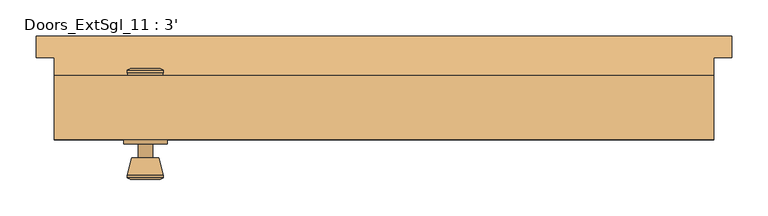
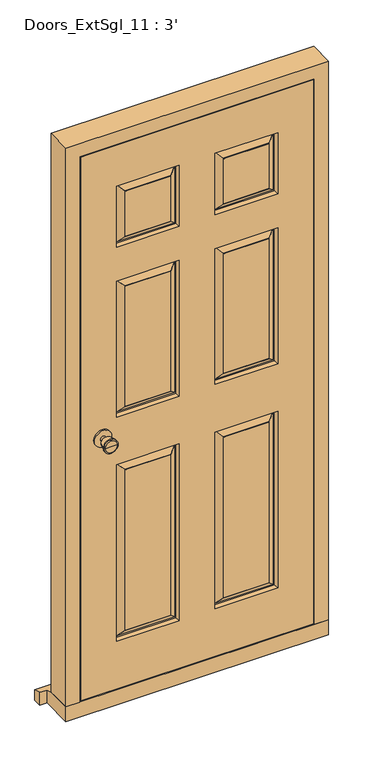
"""IFC4 building model written with IfcOpenShell, lengths in millimetres: door geometry, Doors_ExtSgl_11 : 3'."""

from ifc_helpers import new_model, si_unit, point, frame, frame_2d, origin, place, context, project, spatial, polyline, circle_curve, trimmed, segment, composite_curve, outline, extrude, faceted_brep, source, transform, mapped, element, save
from ifc_brep_helpers import plane_surface, cylinder_surface, revolved_surface, advanced_brep


def doors_extsgl_11_3_cb0934a6(model_context):
    return source(origin(), model_context, "Body", "SolidModel", [
        advanced_brep(
        [(-330.7, -51.42, 1000.0), (-320.7, -51.42, 1000.0), (-340.7, -51.42, 1000.0), (-310.2241324, -100.42, 1000.0), (-330.7, -100.42, 1000.0), (-351.1758676, -100.42, 1000.0), (-305.7, -98.5921319, 1000.0), (-355.7, -98.5921319, 1000.0), (-305.7, -95.1284537, 1000.0), (-355.7, -95.1284537, 1000.0), (-312.063764, -70.42, 1000.0), (-349.336236, -70.42, 1000.0), (-320.7, -70.42, 1000.0), (-340.7, -70.42, 1000.0)],
        [
            (0, 1),
            (1, 2, circle_curve(frame((-330.7, -51.42, 1000.0), z_axis=(0.0, 1.0, 0.0), x_axis=(-1.0, 0.0, 0.0)), 10.0)),
            (2, 0),
            (2, 1, circle_curve(frame((-330.7, -51.42, 1000.0), z_axis=(0.0, 1.0, 0.0), x_axis=(-1.0, 0.0, 0.0)), 10.0)),
            (3, 4),
            (4, 5),
            (5, 3, circle_curve(frame((-330.7, -100.42, 1000.0), z_axis=(0.0, -1.0, 0.0), x_axis=(-1.0, 0.0, 0.0)), 20.4758676)),
            (3, 5, circle_curve(frame((-330.7, -100.42, 1000.0), z_axis=(0.0, -1.0, 0.0), x_axis=(-1.0, 0.0, 0.0)), 20.4758676)),
            (6, 3),
            (5, 7),
            (7, 6, circle_curve(frame((-330.7, -98.5921319, 1000.0), z_axis=(0.0, -1.0, 0.0), x_axis=(-1.0, 0.0, 0.0)), 25.0)),
            (6, 7, circle_curve(frame((-330.7, -98.5921319, 1000.0), z_axis=(0.0, -1.0, 0.0), x_axis=(-1.0, 0.0, 0.0)), 25.0)),
            (8, 6),
            (7, 9),
            (9, 8, circle_curve(frame((-330.7, -95.1284537, 1000.0), z_axis=(0.0, -1.0, 0.0), x_axis=(-1.0, 0.0, 0.0)), 25.0)),
            (8, 9, circle_curve(frame((-330.7, -95.1284537, 1000.0), z_axis=(0.0, -1.0, 0.0), x_axis=(-1.0, 0.0, 0.0)), 25.0)),
            (10, 8),
            (9, 11),
            (11, 10, circle_curve(frame((-330.7, -70.42, 1000.0), z_axis=(0.0, -1.0, 0.0), x_axis=(-1.0, 0.0, 0.0)), 18.636236)),
            (10, 11, circle_curve(frame((-330.7, -70.42, 1000.0), z_axis=(0.0, -1.0, 0.0), x_axis=(-1.0, 0.0, 0.0)), 18.636236)),
            (12, 10),
            (11, 13),
            (13, 12, circle_curve(frame((-330.7, -70.42, 1000.0), z_axis=(0.0, -1.0, 0.0), x_axis=(-1.0, 0.0, 0.0)), 10.0)),
            (12, 13, circle_curve(frame((-330.7, -70.42, 1000.0), z_axis=(0.0, -1.0, 0.0), x_axis=(-1.0, 0.0, 0.0)), 10.0)),
            (1, 12),
            (13, 2),
        ],
        [
            plane_surface(frame((-330.7, -51.42, 1000.0), z_axis=(0.0, 1.0, 0.0), x_axis=(-1.0, 0.0, 0.0))),
            plane_surface(frame((-330.7, -100.42, 1000.0), z_axis=(0.0, -1.0, 0.0), x_axis=(-1.0, 0.0, 0.0))),
            revolved_surface(polyline([(-351.1758676, -100.42, 1000.0), (-355.7, -98.5921319, 1000.0)]), (-330.7, -51.42, 1000.0), (0.0, 1.0, 0.0)),
            cylinder_surface(frame((-330.7, -51.42, 1000.0), z_axis=(0.0, 1.0, 0.0), x_axis=(-1.0, 0.0, 0.0)), 25.0),
            revolved_surface(polyline([(-355.7, -95.1284537, 1000.0), (-349.336236, -70.42, 1000.0)]), (-330.7, -51.42, 1000.0), (0.0, 1.0, 0.0)),
            plane_surface(frame((-330.7, -70.42, 1000.0), z_axis=(0.0, 1.0, 0.0), x_axis=(-1.0, 0.0, 0.0))),
            cylinder_surface(frame((-330.7, -51.42, 1000.0), z_axis=(0.0, 1.0, 0.0), x_axis=(-1.0, 0.0, 0.0)), 10.0),
        ],
        [
            (0, [[1, 2, 3]]),
            (0, [[-3, 4, -1]]),
            (1, [[5, 6, 7]]),
            (1, [[-6, -5, 8]]),
            (2, [[9, -7, 10, 11]]),
            (2, [[-10, -8, -9, 12]]),
            (3, [[13, -11, 14, 15]]),
            (3, [[-14, -12, -13, 16]]),
            (4, [[17, -15, 18, 19]]),
            (4, [[-18, -16, -17, 20]]),
            (5, [[21, -19, 22, 23]]),
            (5, [[-22, -20, -21, 24]]),
            (6, [[25, -23, 26, -2]]),
            (6, [[-26, -24, -25, -4]]),
        ],
    ),
        extrude(outline(composite_curve([segment(trimmed(circle_curve(frame_2d((1000.0, -330.7)), 30.0), [point((1000.0, -360.7))], [point((1000.0, -300.7))], False, "CARTESIAN"), True, "CONTINUOUS"), segment(trimmed(circle_curve(frame_2d((1000.0, -330.7)), 30.0), [point((1000.0, -300.7))], [point((1000.0, -360.7))], False, "CARTESIAN"), True, "CONTINUOUS")], self_intersect=False)), frame((0.0, -51.42, 0.0), z_axis=(0.0, 1.0, 0.0), x_axis=(0.0, 0.0, 1.0)), (0.0, 0.0, 1.0), 6.0),
        advanced_brep(
        [(-330.7, 4.58, 1000.0), (-340.7, 4.58, 1000.0), (-320.7, 4.58, 1000.0), (-310.2241324, 53.58, 1000.0), (-351.1758676, 53.58, 1000.0), (-330.7, 53.58, 1000.0), (-305.7, 51.7521319, 1000.0), (-355.7, 51.7521319, 1000.0), (-305.7, 48.2884537, 1000.0), (-355.7, 48.2884537, 1000.0), (-312.063764, 23.58, 1000.0), (-349.336236, 23.58, 1000.0), (-320.7, 23.58, 1000.0), (-340.7, 23.58, 1000.0)],
        [
            (0, 1),
            (1, 2, circle_curve(frame((-330.7, 4.58, 1000.0), z_axis=(0.0, -1.0, 0.0), x_axis=(-1.0, 0.0, 0.0)), 10.0)),
            (2, 0),
            (2, 1, circle_curve(frame((-330.7, 4.58, 1000.0), z_axis=(0.0, -1.0, 0.0), x_axis=(-1.0, 0.0, 0.0)), 10.0)),
            (3, 4, circle_curve(frame((-330.7, 53.58, 1000.0), z_axis=(0.0, 1.0, 0.0), x_axis=(-1.0, 0.0, 0.0)), 20.4758676)),
            (4, 5),
            (5, 3),
            (4, 3, circle_curve(frame((-330.7, 53.58, 1000.0), z_axis=(0.0, 1.0, 0.0), x_axis=(-1.0, 0.0, 0.0)), 20.4758676)),
            (6, 7, circle_curve(frame((-330.7, 51.7521319, 1000.0), z_axis=(0.0, 1.0, 0.0), x_axis=(-1.0, 0.0, 0.0)), 25.0)),
            (7, 4),
            (3, 6),
            (7, 6, circle_curve(frame((-330.7, 51.7521319, 1000.0), z_axis=(0.0, 1.0, 0.0), x_axis=(-1.0, 0.0, 0.0)), 25.0)),
            (8, 9, circle_curve(frame((-330.7, 48.2884537, 1000.0), z_axis=(0.0, 1.0, 0.0), x_axis=(-1.0, 0.0, 0.0)), 25.0)),
            (9, 7),
            (6, 8),
            (9, 8, circle_curve(frame((-330.7, 48.2884537, 1000.0), z_axis=(0.0, 1.0, 0.0), x_axis=(-1.0, 0.0, 0.0)), 25.0)),
            (10, 11, circle_curve(frame((-330.7, 23.58, 1000.0), z_axis=(0.0, 1.0, 0.0), x_axis=(-1.0, 0.0, 0.0)), 18.636236)),
            (11, 9),
            (8, 10),
            (11, 10, circle_curve(frame((-330.7, 23.58, 1000.0), z_axis=(0.0, 1.0, 0.0), x_axis=(-1.0, 0.0, 0.0)), 18.636236)),
            (12, 13, circle_curve(frame((-330.7, 23.58, 1000.0), z_axis=(0.0, 1.0, 0.0), x_axis=(-1.0, 0.0, 0.0)), 10.0)),
            (13, 11),
            (10, 12),
            (13, 12, circle_curve(frame((-330.7, 23.58, 1000.0), z_axis=(0.0, 1.0, 0.0), x_axis=(-1.0, 0.0, 0.0)), 10.0)),
            (1, 13),
            (12, 2),
        ],
        [
            plane_surface(frame((-330.7, 4.58, 1000.0), z_axis=(0.0, -1.0, 0.0), x_axis=(-1.0, 0.0, 0.0))),
            plane_surface(frame((-330.7, 53.58, 1000.0), z_axis=(0.0, 1.0, 0.0), x_axis=(-1.0, 0.0, 0.0))),
            revolved_surface(polyline([(-351.1758676, 53.58, 1000.0), (-355.7, 51.7521319, 1000.0)]), (-330.7, 4.58, 1000.0), (0.0, -1.0, 0.0)),
            cylinder_surface(frame((-330.7, 4.58, 1000.0), z_axis=(0.0, -1.0, 0.0), x_axis=(-1.0, 0.0, 0.0)), 25.0),
            revolved_surface(polyline([(-355.7, 48.2884537, 1000.0), (-349.336236, 23.58, 1000.0)]), (-330.7, 4.58, 1000.0), (0.0, -1.0, 0.0)),
            plane_surface(frame((-330.7, 23.58, 1000.0), z_axis=(0.0, -1.0, 0.0), x_axis=(-1.0, 0.0, 0.0))),
            cylinder_surface(frame((-330.7, 4.58, 1000.0), z_axis=(0.0, -1.0, 0.0), x_axis=(-1.0, 0.0, 0.0)), 10.0),
        ],
        [
            (0, [[1, 2, 3]]),
            (0, [[-3, 4, -1]]),
            (1, [[5, 6, 7]]),
            (1, [[8, -7, -6]]),
            (2, [[9, 10, -5, 11]]),
            (2, [[12, -11, -8, -10]]),
            (3, [[13, 14, -9, 15]]),
            (3, [[16, -15, -12, -14]]),
            (4, [[17, 18, -13, 19]]),
            (4, [[20, -19, -16, -18]]),
            (5, [[21, 22, -17, 23]]),
            (5, [[24, -23, -20, -22]]),
            (6, [[-2, 25, -21, 26]]),
            (6, [[-4, -26, -24, -25]]),
        ],
    ),
        extrude(outline(composite_curve([segment(trimmed(circle_curve(frame_2d((1000.0, -330.7)), 30.0), [point((1000.0, -360.7))], [point((1000.0, -300.7))], False, "CARTESIAN"), True, "CONTINUOUS"), segment(trimmed(circle_curve(frame_2d((1000.0, -330.7)), 30.0), [point((1000.0, -300.7))], [point((1000.0, -360.7))], False, "CARTESIAN"), True, "CONTINUOUS")], self_intersect=False)), frame((0.0, -1.42, 0.0), z_axis=(0.0, 1.0, 0.0), x_axis=(0.0, 0.0, 1.0)), (0.0, 0.0, 1.0), 6.0),
        faceted_brep([(386.7, 43.58, 54.5), (457.2, 43.58, 54.5), (457.2, -45.42, 54.5), (408.7, -45.42, 54.5), (408.7, 1.58, 54.5), (386.7, 1.58, 54.5), (386.7, 43.58, 2039.5), (-386.7, 43.58, 2039.5), (-386.7, 43.58, 54.5), (-457.2, 43.58, 54.5), (-457.2, 43.58, 2110.0), (457.2, 43.58, 2110.0), (457.2, -45.42, 2110.0), (-457.2, -45.42, 2110.0), (-457.2, -45.42, 54.5), (-408.7, -45.42, 54.5), (-408.7, -45.42, 2061.5), (408.7, -45.42, 2061.5), (408.7, 1.58, 2061.5), (-408.7, 1.58, 2061.5), (-408.7, 1.58, 54.5), (-386.7, 1.58, 54.5), (-386.7, 1.58, 2039.5), (386.7, 1.58, 2039.5)], [[[0, 1, 2, 3, 4, 5]], [[1, 0, 6, 7, 8, 9, 10, 11]], [[2, 1, 11, 12]], [[3, 2, 12, 13, 14, 15, 16, 17]], [[4, 3, 17, 18]], [[5, 4, 18, 19, 20, 21, 22, 23]], [[0, 5, 23, 6]], [[8, 7, 22, 21]], [[9, 8, 21, 20, 15, 14]], [[10, 9, 14, 13]], [[16, 15, 20, 19]], [[11, 10, 13, 12]], [[17, 16, 19, 18]], [[7, 6, 23, 22]]]),
        faceted_brep([(405.7, -45.42, 58.5), (405.7, -45.42, 2058.5), (-406.6250294, -45.42, 2058.5), (-406.6250294, -45.42, 58.5), (-62.5, -45.42, 883.5), (-62.5, -45.42, 233.5), (-280.7, -45.42, 233.5), (-280.7, -45.42, 883.5), (280.7, -45.42, 883.5), (280.7, -45.42, 233.5), (62.5, -45.42, 233.5), (62.5, -45.42, 883.5), (-62.5, -45.42, 1558.5), (-62.5, -45.42, 1058.5), (-280.7, -45.42, 1058.5), (-280.7, -45.42, 1558.5), (280.7, -45.42, 1558.5), (280.7, -45.42, 1058.5), (62.5, -45.42, 1058.5), (62.5, -45.42, 1558.5), (-62.5, -45.42, 1908.5), (-62.5, -45.42, 1683.5), (-280.7, -45.42, 1683.5), (-280.7, -45.42, 1908.5), (62.5, -45.42, 1683.5), (62.5, -45.42, 1908.5), (280.7, -45.42, 1908.5), (280.7, -45.42, 1683.5), (-92.5, -45.42, 263.5), (-92.5, -45.42, 853.5), (-250.7, -45.42, 853.5), (-250.7, -45.42, 263.5), (250.7, -45.42, 263.5), (250.7, -45.42, 853.5), (92.5, -45.42, 853.5), (92.5, -45.42, 263.5), (-92.5, -45.42, 1088.5), (-92.5, -45.42, 1528.5), (-250.7, -45.42, 1528.5), (-250.7, -45.42, 1088.5), (250.7, -45.42, 1088.5), (250.7, -45.42, 1528.5), (92.5, -45.42, 1528.5), (92.5, -45.42, 1088.5), (-92.5, -45.42, 1713.5), (-92.5, -45.42, 1878.5), (-250.7, -45.42, 1878.5), (-250.7, -45.42, 1713.5), (92.5, -45.42, 1878.5), (92.5, -45.42, 1713.5), (250.7, -45.42, 1713.5), (250.7, -45.42, 1878.5), (405.7, -1.42, 58.5), (-406.6250294, -1.42, 58.5), (-406.6250294, -1.42, 2058.5), (405.7, -1.42, 2058.5), (62.5, -1.42, 883.5), (62.5, -1.42, 233.5), (280.7, -1.42, 233.5), (280.7, -1.42, 883.5), (-280.7, -1.42, 883.5), (-280.7, -1.42, 233.5), (-62.5, -1.42, 233.5), (-62.5, -1.42, 883.5), (62.5, -1.42, 1558.5), (62.5, -1.42, 1058.5), (280.7, -1.42, 1058.5), (280.7, -1.42, 1558.5), (-280.7, -1.42, 1558.5), (-280.7, -1.42, 1058.5), (-62.5, -1.42, 1058.5), (-62.5, -1.42, 1558.5), (62.5, -1.42, 1908.5), (62.5, -1.42, 1683.5), (280.7, -1.42, 1683.5), (280.7, -1.42, 1908.5), (-280.7, -1.42, 1908.5), (-280.7, -1.42, 1683.5), (-62.5, -1.42, 1683.5), (-62.5, -1.42, 1908.5), (92.5, -1.42, 263.5), (92.5, -1.42, 853.5), (250.7, -1.42, 853.5), (250.7, -1.42, 263.5), (-250.7, -1.42, 263.5), (-250.7, -1.42, 853.5), (-92.5, -1.42, 853.5), (-92.5, -1.42, 263.5), (92.5, -1.42, 1088.5), (92.5, -1.42, 1528.5), (250.7, -1.42, 1528.5), (250.7, -1.42, 1088.5), (-250.7, -1.42, 1088.5), (-250.7, -1.42, 1528.5), (-92.5, -1.42, 1528.5), (-92.5, -1.42, 1088.5), (92.5, -1.42, 1713.5), (92.5, -1.42, 1878.5), (250.7, -1.42, 1878.5), (250.7, -1.42, 1713.5), (-250.7, -1.42, 1713.5), (-250.7, -1.42, 1878.5), (-92.5, -1.42, 1878.5), (-92.5, -1.42, 1713.5), (65.5, -16.42, 880.5), (65.5, -16.42, 236.5), (90.5, -2.42, 855.5), (90.5, -2.42, 261.5), (70.5, -16.42, 241.5), (70.5, -16.42, 875.5), (92.5, -2.42, 263.5), (92.5, -2.42, 853.5), (277.7, -16.42, 236.5), (252.7, -2.42, 261.5), (272.7, -16.42, 241.5), (250.7, -2.42, 263.5), (277.7, -16.42, 880.5), (252.7, -2.42, 855.5), (272.7, -16.42, 875.5), (250.7, -2.42, 853.5), (-277.7, -16.42, 880.5), (-277.7, -16.42, 236.5), (-252.7, -2.42, 855.5), (-252.7, -2.42, 261.5), (-272.7, -16.42, 241.5), (-272.7, -16.42, 875.5), (-250.7, -2.42, 263.5), (-250.7, -2.42, 853.5), (-65.5, -16.42, 236.5), (-90.5, -2.42, 261.5), (-70.5, -16.42, 241.5), (-92.5, -2.42, 263.5), (-65.5, -16.42, 880.5), (-90.5, -2.42, 855.5), (-70.5, -16.42, 875.5), (-92.5, -2.42, 853.5), (-92.5, -44.42, 263.5), (-92.5, -44.42, 853.5), (-70.5, -30.42, 241.5), (-70.5, -30.42, 875.5), (-90.5, -44.42, 855.5), (-90.5, -44.42, 261.5), (-65.5, -30.42, 880.5), (-65.5, -30.42, 236.5), (-250.7, -44.42, 853.5), (-272.7, -30.42, 875.5), (-252.7, -44.42, 855.5), (-277.7, -30.42, 880.5), (-250.7, -44.42, 263.5), (-272.7, -30.42, 241.5), (-252.7, -44.42, 261.5), (-277.7, -30.42, 236.5), (277.7, -30.42, 880.5), (277.7, -30.42, 236.5), (252.7, -44.42, 855.5), (252.7, -44.42, 261.5), (272.7, -30.42, 241.5), (272.7, -30.42, 875.5), (250.7, -44.42, 263.5), (250.7, -44.42, 853.5), (65.5, -30.42, 236.5), (90.5, -44.42, 261.5), (70.5, -30.42, 241.5), (92.5, -44.42, 263.5), (65.5, -30.42, 880.5), (90.5, -44.42, 855.5), (70.5, -30.42, 875.5), (92.5, -44.42, 853.5), (92.5, -2.42, 1088.5), (92.5, -2.42, 1528.5), (70.5, -16.42, 1066.5), (70.5, -16.42, 1550.5), (90.5, -2.42, 1530.5), (90.5, -2.42, 1086.5), (65.5, -16.42, 1555.5), (65.5, -16.42, 1061.5), (250.7, -2.42, 1528.5), (272.7, -16.42, 1550.5), (252.7, -2.42, 1530.5), (277.7, -16.42, 1555.5), (250.7, -2.42, 1088.5), (272.7, -16.42, 1066.5), (252.7, -2.42, 1086.5), (277.7, -16.42, 1061.5), (-250.7, -2.42, 1088.5), (-250.7, -2.42, 1528.5), (-272.7, -16.42, 1066.5), (-272.7, -16.42, 1550.5), (-252.7, -2.42, 1530.5), (-252.7, -2.42, 1086.5), (-277.7, -16.42, 1555.5), (-277.7, -16.42, 1061.5), (-92.5, -2.42, 1528.5), (-70.5, -16.42, 1550.5), (-90.5, -2.42, 1530.5), (-65.5, -16.42, 1555.5), (-92.5, -2.42, 1088.5), (-70.5, -16.42, 1066.5), (-90.5, -2.42, 1086.5), (-65.5, -16.42, 1061.5), (-92.5, -44.42, 1088.5), (-92.5, -44.42, 1528.5), (-70.5, -30.42, 1066.5), (-70.5, -30.42, 1550.5), (-90.5, -44.42, 1530.5), (-90.5, -44.42, 1086.5), (-65.5, -30.42, 1555.5), (-65.5, -30.42, 1061.5), (-250.7, -44.42, 1528.5), (-272.7, -30.42, 1550.5), (-252.7, -44.42, 1530.5), (-277.7, -30.42, 1555.5), (-250.7, -44.42, 1088.5), (-272.7, -30.42, 1066.5), (-252.7, -44.42, 1086.5), (-277.7, -30.42, 1061.5), (277.7, -30.42, 1555.5), (277.7, -30.42, 1061.5), (252.7, -44.42, 1530.5), (252.7, -44.42, 1086.5), (272.7, -30.42, 1066.5), (272.7, -30.42, 1550.5), (250.7, -44.42, 1088.5), (250.7, -44.42, 1528.5), (65.5, -30.42, 1061.5), (90.5, -44.42, 1086.5), (70.5, -30.42, 1066.5), (92.5, -44.42, 1088.5), (65.5, -30.42, 1555.5), (90.5, -44.42, 1530.5), (70.5, -30.42, 1550.5), (92.5, -44.42, 1528.5), (92.5, -2.42, 1713.5), (92.5, -2.42, 1878.5), (70.5, -16.42, 1691.5), (70.5, -16.42, 1900.5), (90.5, -2.42, 1880.5), (90.5, -2.42, 1711.5), (65.5, -16.42, 1905.5), (65.5, -16.42, 1686.5), (250.7, -2.42, 1878.5), (272.7, -16.42, 1900.5), (252.7, -2.42, 1880.5), (277.7, -16.42, 1905.5), (250.7, -2.42, 1713.5), (272.7, -16.42, 1691.5), (252.7, -2.42, 1711.5), (277.7, -16.42, 1686.5), (-250.7, -2.42, 1713.5), (-250.7, -2.42, 1878.5), (-272.7, -16.42, 1691.5), (-272.7, -16.42, 1900.5), (-252.7, -2.42, 1880.5), (-252.7, -2.42, 1711.5), (-277.7, -16.42, 1905.5), (-277.7, -16.42, 1686.5), (-92.5, -2.42, 1878.5), (-70.5, -16.42, 1900.5), (-90.5, -2.42, 1880.5), (-65.5, -16.42, 1905.5), (-92.5, -2.42, 1713.5), (-70.5, -16.42, 1691.5), (-90.5, -2.42, 1711.5), (-65.5, -16.42, 1686.5), (-92.5, -44.42, 1713.5), (-92.5, -44.42, 1878.5), (-70.5, -30.42, 1691.5), (-70.5, -30.42, 1900.5), (-90.5, -44.42, 1880.5), (-90.5, -44.42, 1711.5), (-65.5, -30.42, 1905.5), (-65.5, -30.42, 1686.5), (-250.7, -44.42, 1878.5), (-272.7, -30.42, 1900.5), (-252.7, -44.42, 1880.5), (-277.7, -30.42, 1905.5), (-250.7, -44.42, 1713.5), (-272.7, -30.42, 1691.5), (-252.7, -44.42, 1711.5), (-277.7, -30.42, 1686.5), (92.5, -44.42, 1878.5), (92.5, -44.42, 1713.5), (70.5, -30.42, 1900.5), (70.5, -30.42, 1691.5), (90.5, -44.42, 1711.5), (90.5, -44.42, 1880.5), (65.5, -30.42, 1686.5), (65.5, -30.42, 1905.5), (250.7, -44.42, 1713.5), (272.7, -30.42, 1691.5), (252.7, -44.42, 1711.5), (277.7, -30.42, 1686.5), (250.7, -44.42, 1878.5), (272.7, -30.42, 1900.5), (252.7, -44.42, 1880.5), (277.7, -30.42, 1905.5)], [[[0, 1, 2, 3], [4, 5, 6, 7], [8, 9, 10, 11], [12, 13, 14, 15], [16, 17, 18, 19], [20, 21, 22, 23], [24, 25, 26, 27]], [[28, 29, 30, 31]], [[32, 33, 34, 35]], [[36, 37, 38, 39]], [[40, 41, 42, 43]], [[44, 45, 46, 47]], [[48, 49, 50, 51]], [[52, 53, 54, 55], [56, 57, 58, 59], [60, 61, 62, 63], [64, 65, 66, 67], [68, 69, 70, 71], [72, 73, 74, 75], [76, 77, 78, 79]], [[80, 81, 82, 83]], [[84, 85, 86, 87]], [[88, 89, 90, 91]], [[92, 93, 94, 95]], [[96, 97, 98, 99]], [[100, 101, 102, 103]], [[1, 0, 52, 55]], [[2, 1, 55, 54]], [[3, 2, 54, 53]], [[0, 3, 53, 52]], [[104, 105, 57, 56]], [[106, 107, 108, 109]], [[80, 110, 111, 81]], [[57, 105, 112, 58]], [[108, 107, 113, 114]], [[110, 80, 83, 115]], [[58, 112, 116, 59]], [[114, 113, 117, 118]], [[115, 83, 82, 119]], [[104, 56, 59, 116]], [[105, 104, 116, 112], [109, 108, 114, 118]], [[106, 109, 118, 117]], [[107, 106, 117, 113], [111, 110, 115, 119]], [[81, 111, 119, 82]], [[120, 121, 61, 60]], [[122, 123, 124, 125]], [[84, 126, 127, 85]], [[61, 121, 128, 62]], [[124, 123, 129, 130]], [[126, 84, 87, 131]], [[62, 128, 132, 63]], [[130, 129, 133, 134]], [[131, 87, 86, 135]], [[120, 60, 63, 132]], [[121, 120, 132, 128], [125, 124, 130, 134]], [[122, 125, 134, 133]], [[123, 122, 133, 129], [127, 126, 131, 135]], [[85, 127, 135, 86]], [[136, 137, 29, 28]], [[138, 139, 140, 141]], [[4, 142, 143, 5]], [[29, 137, 144, 30]], [[140, 139, 145, 146]], [[142, 4, 7, 147]], [[30, 144, 148, 31]], [[146, 145, 149, 150]], [[147, 7, 6, 151]], [[136, 28, 31, 148]], [[141, 140, 146, 150], [137, 136, 148, 144]], [[138, 141, 150, 149]], [[143, 142, 147, 151], [139, 138, 149, 145]], [[5, 143, 151, 6]], [[152, 153, 9, 8]], [[154, 155, 156, 157]], [[32, 158, 159, 33]], [[9, 153, 160, 10]], [[156, 155, 161, 162]], [[158, 32, 35, 163]], [[10, 160, 164, 11]], [[162, 161, 165, 166]], [[163, 35, 34, 167]], [[152, 8, 11, 164]], [[153, 152, 164, 160], [157, 156, 162, 166]], [[154, 157, 166, 165]], [[155, 154, 165, 161], [159, 158, 163, 167]], [[33, 159, 167, 34]], [[168, 169, 89, 88]], [[170, 171, 172, 173]], [[64, 174, 175, 65]], [[89, 169, 176, 90]], [[172, 171, 177, 178]], [[174, 64, 67, 179]], [[90, 176, 180, 91]], [[178, 177, 181, 182]], [[179, 67, 66, 183]], [[168, 88, 91, 180]], [[173, 172, 178, 182], [169, 168, 180, 176]], [[170, 173, 182, 181]], [[175, 174, 179, 183], [171, 170, 181, 177]], [[65, 175, 183, 66]], [[184, 185, 93, 92]], [[186, 187, 188, 189]], [[68, 190, 191, 69]], [[93, 185, 192, 94]], [[188, 187, 193, 194]], [[190, 68, 71, 195]], [[94, 192, 196, 95]], [[194, 193, 197, 198]], [[195, 71, 70, 199]], [[184, 92, 95, 196]], [[189, 188, 194, 198], [185, 184, 196, 192]], [[186, 189, 198, 197]], [[191, 190, 195, 199], [187, 186, 197, 193]], [[69, 191, 199, 70]], [[200, 201, 37, 36]], [[202, 203, 204, 205]], [[12, 206, 207, 13]], [[37, 201, 208, 38]], [[204, 203, 209, 210]], [[206, 12, 15, 211]], [[38, 208, 212, 39]], [[210, 209, 213, 214]], [[211, 15, 14, 215]], [[200, 36, 39, 212]], [[205, 204, 210, 214], [201, 200, 212, 208]], [[202, 205, 214, 213]], [[207, 206, 211, 215], [203, 202, 213, 209]], [[13, 207, 215, 14]], [[216, 217, 17, 16]], [[218, 219, 220, 221]], [[40, 222, 223, 41]], [[17, 217, 224, 18]], [[220, 219, 225, 226]], [[222, 40, 43, 227]], [[18, 224, 228, 19]], [[226, 225, 229, 230]], [[227, 43, 42, 231]], [[216, 16, 19, 228]], [[217, 216, 228, 224], [221, 220, 226, 230]], [[218, 221, 230, 229]], [[219, 218, 229, 225], [223, 222, 227, 231]], [[41, 223, 231, 42]], [[232, 233, 97, 96]], [[234, 235, 236, 237]], [[72, 238, 239, 73]], [[97, 233, 240, 98]], [[236, 235, 241, 242]], [[238, 72, 75, 243]], [[98, 240, 244, 99]], [[242, 241, 245, 246]], [[243, 75, 74, 247]], [[232, 96, 99, 244]], [[237, 236, 242, 246], [233, 232, 244, 240]], [[234, 237, 246, 245]], [[239, 238, 243, 247], [235, 234, 245, 241]], [[73, 239, 247, 74]], [[248, 249, 101, 100]], [[250, 251, 252, 253]], [[76, 254, 255, 77]], [[101, 249, 256, 102]], [[252, 251, 257, 258]], [[254, 76, 79, 259]], [[102, 256, 260, 103]], [[258, 257, 261, 262]], [[259, 79, 78, 263]], [[248, 100, 103, 260]], [[253, 252, 258, 262], [249, 248, 260, 256]], [[250, 253, 262, 261]], [[255, 254, 259, 263], [251, 250, 261, 257]], [[77, 255, 263, 78]], [[264, 265, 45, 44]], [[266, 267, 268, 269]], [[20, 270, 271, 21]], [[45, 265, 272, 46]], [[268, 267, 273, 274]], [[270, 20, 23, 275]], [[46, 272, 276, 47]], [[274, 273, 277, 278]], [[275, 23, 22, 279]], [[264, 44, 47, 276]], [[269, 268, 274, 278], [265, 264, 276, 272]], [[266, 269, 278, 277]], [[271, 270, 275, 279], [267, 266, 277, 273]], [[21, 271, 279, 22]], [[280, 281, 49, 48]], [[282, 283, 284, 285]], [[24, 286, 287, 25]], [[49, 281, 288, 50]], [[284, 283, 289, 290]], [[286, 24, 27, 291]], [[50, 288, 292, 51]], [[290, 289, 293, 294]], [[291, 27, 26, 295]], [[280, 48, 51, 292]], [[285, 284, 290, 294], [281, 280, 292, 288]], [[282, 285, 294, 293]], [[287, 286, 291, 295], [283, 282, 293, 289]], [[25, 287, 295, 26]]]),
        faceted_brep([(482.2, 98.58, 0.0), (482.2, 98.58, 38.5947221), (482.2, 68.58, 47.2703282), (482.2, 68.58, 0.0), (-482.2, 98.58, 38.5947221), (-482.2, 98.58, 0.0), (-482.2, 68.58, 0.0), (-482.2, 68.58, 47.2703282), (457.2, 68.58, 0.0), (457.2, -45.42, 0.0), (-457.2, -45.42, 0.0), (-457.2, 68.58, 0.0), (-457.2, 68.58, 47.2703282), (-457.2, 43.58, 54.5), (457.2, 43.58, 54.5), (457.2, 68.58, 47.2703282), (-457.2, -45.42, 54.5), (457.2, -45.42, 54.5)], [[[0, 1, 2, 3]], [[4, 5, 6, 7]], [[5, 0, 3, 8, 9, 10, 11, 6]], [[1, 0, 5, 4]], [[1, 4, 7, 12, 13, 14, 15, 2]], [[13, 16, 17, 14]], [[16, 10, 9, 17]], [[12, 11, 10, 16, 13]], [[11, 12, 7, 6]], [[8, 15, 14, 17, 9]], [[15, 8, 3, 2]]]),
    ])


if __name__ == "__main__":
    model = new_model("IFC4")
    model_context = context("Model", 3, world=origin())
    ifc_project = project(units=[si_unit("LENGTHUNIT", "METRE", prefix="MILLI")], contexts=[model_context])
    site = spatial("IfcSite", under=ifc_project)
    building = spatial("IfcBuilding", under=site)
    placement = place(None, origin())
    doors_extsgl_11_3_shape = doors_extsgl_11_3_cb0934a6(model_context)
    element("IfcDoor", 1, ObjectType="Doors_ExtSgl_11 : 3'", at=placement, inside=building, context=model_context, shape_type="MappedRepresentation", body=[
        mapped(doors_extsgl_11_3_shape, transform((0.0, 0.0, 0.0), x_axis=(1.0, 0.0, 0.0), y_axis=(0.0, 1.0, 0.0), z_axis=(0.0, 0.0, 1.0))),
    ])
    save(model, "model.ifc")

# Revit data of these elements
# Type "Doors_ExtSgl_11 : 3'"
#   Type Mark = "49"
#   Type Comments = "External Single"
#   Operation = "SingleSwingRight"
#   Construction Type Id = "MDOOR"
#   Keynote = "L20"
#   Analytic Construction = "Metal"
#   Wrap Layers (Int) from Ext = 177.5 mm
#   Wrap Layers (Ext) from Ext = 102.5 mm
#   Thickness = 44 mm
#   Stile Top of Lock rail = 1000 mm
#   Stile Top of Frieze Rail = 1625 mm
#   Stile Top Rail = 150 mm
#   Stile Shutting = 125 mm
#   Stile Muntin Rail = 125 mm
#   Stile Lock Rail = 175 mm
#   Stile Intermediate/Frieze = 125 mm
#   Stile Hanging = 125 mm
#   Stile Bottom Rail = 175 mm
#   Rough Width = 914.4 mm
#   Rough Height = 2110 mm
#   O/A Frame Width = 64 mm
#   Heat Transfer Coefficient (U) = 3.7021 W/(m²·K)
#   Handle Z Distance = 1000 mm
#   Glazing Thickness = 24 mm
#   FrameWidth = 42 mm
#   FrameOffset - External = 25 mm
#   FrameDepth = 89 mm
#   Door Panel Width = 811.4 mm
#   Door Panel Thickness = 44 mm
#   Door Panel Height = 2000 mm
#   Cill Thickness = 54.5 mm
#   Handle X Distance = 75 mm
#   Height = 2110 mm
#   Structural Tolerance = 6.5 mm
#   Tolerance = 3 mm
#   Undercut = 4 mm
#   Width = 914.4 mm
#   Cill Projection = 30 mm
#   Cill Extension = 25 mm
#   Cavity Closer Width = 50 mm
#   Cavity Closer Offset from Ext = 102.5 mm
#   Cavity Closer Depth = 85 mm
#   Vis - Ironmongery = yes
#   Vis - Cavity Closers = yes
#   Define Thermal Properties by = 1
#   Function = 1
#   Material Door = Door - Panel
#   Material Frame = Door - Frame/Mullion
#   Material Ironmongery = Door - Handle
#   Visual Light Transmittance = 0
#   Solar Heat Gain Coefficient = 0
#   Wall Closure = (empty or 0)
# Element 1 (IfcDoor, "Doors_ExtSgl_11 : 3'")
#   Materials on its faces: "Door - Panel", "Door - Handle", "Door - Frame/Mullion"
# Materials
#   "Door - Panel": class "Wood", colour RGB 210 159 95, transparency 0, Keynote = "L20", Cost = 0
#   "Door - Frame/Mullion": class "Wood", colour RGB 212 179 113, transparency 0, Keynote = "L20", Cost = 0
#   "Door - Handle": colour RGB 0 0 0, transparency 0, Keynote = "P21", Cost = 0
